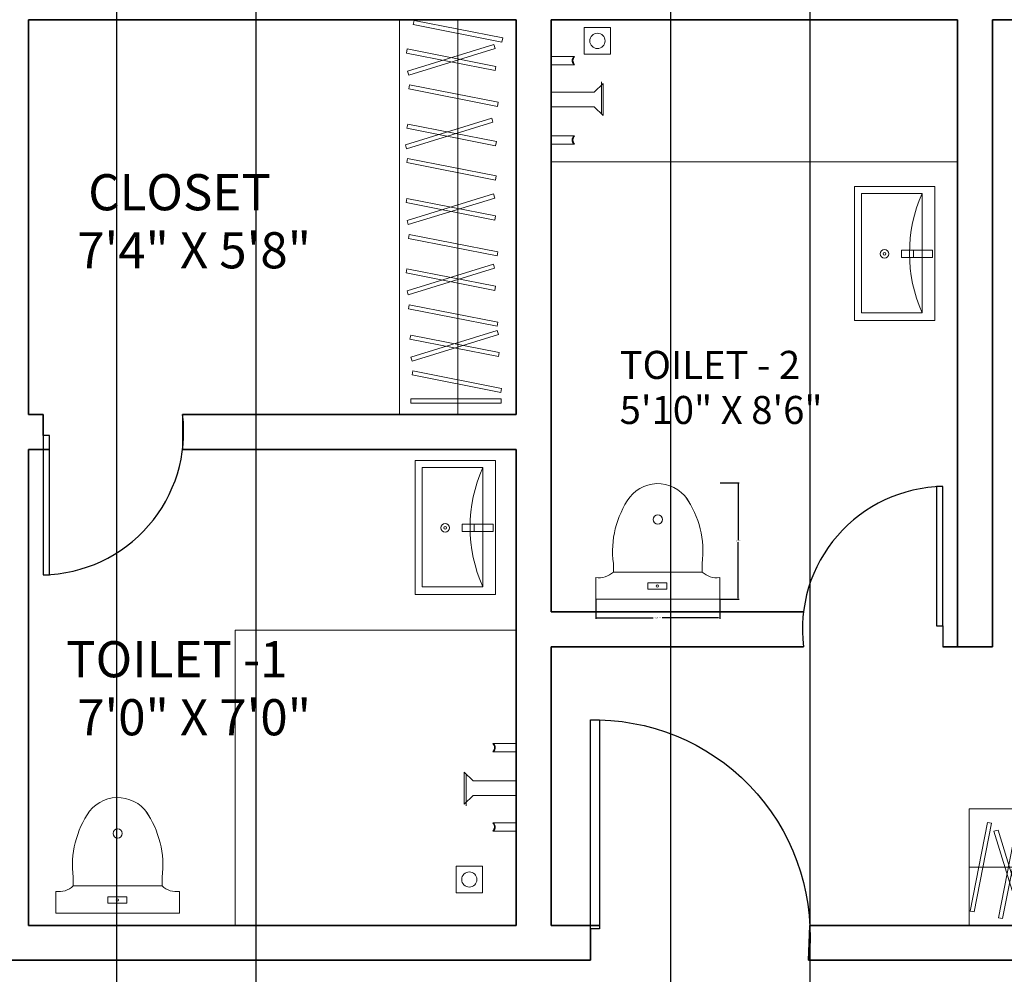
# Model space of a CAD drawing. Units: inches. Extents: x -61 to 1599, y -1316 to 257.
# Tile 141 of 204: x 236 to 406, y -16 to 149. Entities that reach past the tile are written whole.
import ezdxf

# ---------------------------------------------------------------- set-up
doc = ezdxf.new("R2010")
doc.units = ezdxf.units.IN
doc.header["$MEASUREMENT"] = 0
doc.linetypes.add('ACAD_ISO02W100', pattern=[15, 12, -3])
for name, color, linetype, lineweight in [('A-ANNO-DIMS', 2, 'Continuous', 18), ('A-AREA-IDEN', 1, 'Continuous', 18), ('A-FLOR-CASE', 8, 'Continuous', 18), ('A-FLOR-FIXT', 8, 'Continuous', 18), ('A-WALL-JAMB', 4, 'ACAD_ISO02W100', 25), ('DOORS', 2, 'Continuous', 25), ('WALLS', 4, 'Continuous', 35)]:
    doc.layers.add(name, color=color, linetype=linetype, lineweight=lineweight)
doc.styles.get("Standard").update_dxf_attribs({"font": 'arial.ttf'})
doc.dimstyles.get("Standard").update_dxf_attribs({"dimtxt": 0.18, "dimasz": 0.18, "dimexe": 0.18, "dimexo": 0.0625, "dimgap": 0.09, "dimtad": 0, "dimtih": 1, "dimtoh": 1, "dimdec": 0, "dimzin": 0, "dimdsep": 46, "dimlunit": 3, "dimtxsty": 'Standard', "dimcen": 0.09, "dimadec": 0, "dimazin": 0, "dimtfac": 1, "dimtdec": 0, "dimtofl": 0, "dimtmove": 0, "dimatfit": 3, "dimfxl": 1, "dimtolj": 1, "dimtzin": 0, "dimarcsym": 0})

# ---------------------------------------------------------------- blocks, each defined once
blk = doc.blocks.new('DOOR-SWING-24')
blk.add_line((0, 0), (0, 3.6))
blk.add_lwpolyline([(0, 0), (0, -24), (1.05, -24), (1.05, 0)], close=True)
blk.add_arc((-0.44, 0.62), 24.62, 271.0259, 6.9559)
blk = doc.blocks.new('DOOR-SWING-36')
blk.add_line((0, 0), (0, -5.4))
blk.add_lwpolyline([(0, 0), (0, 36), (-1.57, 36), (-1.57, 0)], close=True)
blk.add_arc((-0.74, -1.08), 37.09, 91.2913, 186.6905)
blk = doc.blocks.new('WC-FLOOR-MOUNT')
for p, q in [((3.02, 4.69), (3.02, 6.17)), ((18.31, 4.69), (18.31, 6.17)), ((0, 0), (0, 3.75)), ((3.02, 4.69), (18.31, 4.69)), ((21.33, 0), (21.33, 3.75)), ((0, 0), (21.33, 0))]:
    blk.add_line(p, q)
blk.add_lwpolyline([(12.24, 1.73), (8.96, 1.73), (8.96, 2.81), (12.24, 2.81)], close=True)
for centre, radius in [((10.67, 13.73), 0.792), ((10.6, 2.27), 0.208)]:
    blk.add_circle(centre, radius)
for centre, radius, start, end in [((10.67, 13.73), 6.18, 27.6844, 141.4697), ((19.05, 8.26), 16.17, 144.824, 187.4232), ((2.28, 8.26), 16.17, 352.5768, 35.176), ((0.56, 7.25), 3.55, 260.8586, 313.6993), ((20.77, 7.25), 3.55, 226.3007, 279.1414)]:
    blk.add_arc(centre, radius, start, end)
blk = doc.blocks.new('LAVATORY-WALL')
blk.add_line((10.19, 12.11), (10.19, 10.88))
for points in [[(13.87, 0), (0, 0), (0, 23.07), (13.87, 23.07)], [(13.87, 0), (0, 0), (0, 23.07), (13.87, 23.07)], [(1.2, 1.34), (1.2, 21.88), (11.67, 21.88), (11.67, 1.34)], [(8.09, 10.88), (8.09, 12.11), (13.47, 12.11), (13.47, 10.88)]]:
    blk.add_lwpolyline(points, close=True)
for radius in [0.74, 0.233]:
    blk.add_circle((5.16, 11.5), radius)
blk.add_arc((34.73, 11.61), 25.25, 155.9939, 204.0061)
blk = doc.blocks.new('SHOWER-FITTINGS')
for p, q in [((10.35, 25.72), (6.31, 25.72)), ((10.35, 24.3), (6.31, 24.3)), ((10.35, 23), (10.35, 23)), ((2.92, 19.29), (1.4, 20.76)), ((1.4, 15.27), (1.4, 20.76)), ((1.69, 14.98), (1.69, 20.48)), ((10.35, 19.29), (2.92, 19.29)), ((2.92, 16.74), (1.4, 15.27)), ((10.35, 16.74), (2.92, 16.74)), ((10.35, 12.03), (6.31, 12.03)), ((10.35, 10.61), (6.31, 10.61))]:
    blk.add_line(p, q)
blk.add_lwpolyline([(4.52, 0), (0, 0), (0, 4.57), (4.52, 4.57)], close=True)
blk.add_circle((2.26, 2.29), 1.31)
for points in [[(6.31, 24.3), (6.45, 24.53), (6.75, 25), (6.46, 25.48), (6.31, 25.72)], [(6.45, 24.3), (6.59, 24.53), (6.88, 25), (6.59, 25.48), (6.45, 25.72)], [(6.31, 10.61), (6.45, 10.84), (6.75, 11.31), (6.46, 11.78), (6.31, 12.03)], [(6.45, 10.61), (6.59, 10.84), (6.88, 11.31), (6.59, 11.78), (6.45, 12.03)]]:
    blk.add_open_spline(points, degree=3, knots=[0, 0, 0, 0, 0.7501, 1.532449, 1.532449, 1.532449, 1.532449])
blk = doc.blocks.new('SHOWER-FITTINGS-2')
for p, q in [((0, 15.11), (4.04, 15.11)), ((0, 13.69), (4.04, 13.69)), ((7.43, 8.98), (8.95, 10.45)), ((8.66, 10.73), (8.66, 5.24)), ((8.95, 10.45), (8.95, 4.96)), ((0, 8.98), (7.43, 8.98)), ((0, 6.43), (7.43, 6.43)), ((7.43, 6.43), (8.95, 4.96)), ((0, 1.42), (4.04, 1.42)), ((0, 0), (4.04, 0))]:
    blk.add_line(p, q)
blk.add_lwpolyline([(10.23, 15.5), (5.71, 15.5), (5.71, 20.08), (10.23, 20.08)], close=True)
blk.add_circle((7.97, 17.79), 1.31)
for points in [[(3.91, 15.11), (3.76, 14.88), (3.47, 14.41), (3.76, 13.94), (3.91, 13.69)], [(4.04, 15.11), (3.9, 14.88), (3.6, 14.41), (3.89, 13.94), (4.04, 13.69)], [(3.91, 1.42), (3.76, 1.19), (3.47, 0.72), (3.76, 0.24), (3.91, 0)], [(4.04, 1.42), (3.9, 1.19), (3.6, 0.72), (3.89, 0.24), (4.04, 0)]]:
    blk.add_open_spline(points, degree=3, knots=[0, 0, 0, 0, 0.7501, 1.532449, 1.532449, 1.532449, 1.532449])
blk = doc.blocks.new('WARDROBE-HANGING')
blk.add_line((10.05, 0), (10.05, 68))
for points in [[(20.09, 0), (0, 0), (0, 68), (20.09, 68)], [(2.48, 67.85), (17.75, 64.85), (17.61, 64.14), (2.34, 67.15)], [(1.32, 62.96), (16.59, 59.95), (16.45, 59.25), (1.19, 62.25)], [(1.35, 59.16), (16.22, 63.73), (16.43, 63.04), (1.56, 58.47)], [(1.71, 56.78), (16.98, 53.78), (16.84, 53.07), (1.57, 56.08)], [(1, 46.47), (15.87, 51.04), (16.08, 50.35), (1.21, 45.78)], [(1.39, 50.01), (16.66, 47.01), (16.52, 46.3), (1.26, 49.31)], [(1.36, 44.09), (16.63, 41.09), (16.49, 40.38), (1.23, 43.38)], [(1.28, 33.41), (16.16, 37.98), (16.37, 37.29), (1.49, 32.72)], [(1.26, 37.2), (16.53, 34.2), (16.39, 33.49), (1.12, 36.5)], [(1.65, 31.03), (16.92, 28.03), (16.78, 27.32), (1.51, 30.32)], [(1.28, 21.3), (16.15, 25.87), (16.36, 25.18), (1.49, 20.61)], [(1.26, 25.09), (16.53, 22.09), (16.39, 21.38), (1.12, 24.39)], [(1.65, 18.92), (16.91, 15.92), (16.78, 15.21), (1.51, 18.21)], [(1.91, 13.69), (17.17, 10.68), (17.04, 9.98), (1.77, 12.98)], [(1.93, 9.89), (16.8, 14.46), (17.01, 13.77), (2.14, 9.2)], [(2.29, 7.51), (17.56, 4.51), (17.42, 3.8), (2.16, 6.81)], [(17.49, 1.96), (1.93, 1.96), (1.93, 2.68), (17.49, 2.68)]]:
    blk.add_lwpolyline(points, close=True)
blk = doc.blocks.new('*D616')
at = {"layer": 'A-ANNO-DIMS', "color": 0, "lineweight": -2, "transparency": 16777216}
for p, q in [((335.4, 48.8), (335.4, 45.48)), ((356.73, 48.8), (356.73, 45.48)), ((335.58, 45.66), (345.29, 45.66)), ((356.55, 45.66), (346.84, 45.66))]:
    blk.add_line(p, q, dxfattribs=at)
at = {"layer": 'A-ANNO-DIMS', "color": 0, "transparency": 16777216}
for points in [[(335.58, 45.69), (335.58, 45.63), (335.4, 45.66)], [(356.55, 45.69), (356.55, 45.63), (356.73, 45.66)]]:
    blk.add_solid(points, dxfattribs=at)
at = {"layer": 'DEFPOINTS', "color": 0, "transparency": 16777216}
for p in [(335.4, 48.86), (356.73, 48.86), (356.73, 45.66)]:
    blk.add_point(p, dxfattribs=at)
at = {"layer": 'A-ANNO-DIMS', "color": 0, "transparency": 16777216, "insert": (346.07, 45.66), "char_height": 0.18, "attachment_point": 5}
blk.add_mtext('\\A1;WC 21 TYP.', dxfattribs=at)
blk = doc.blocks.new('*D617')
at = {"layer": 'A-ANNO-DIMS', "color": 0, "lineweight": -2, "transparency": 16777216}
for p, q in [((356.8, 68.94), (360.11, 68.94)), ((359.93, 68.76), (359.93, 59.08)), ((359.93, 49.04), (359.93, 58.72)), ((356.8, 48.86), (360.11, 48.86))]:
    blk.add_line(p, q, dxfattribs=at)
at = {"layer": 'A-ANNO-DIMS', "color": 0, "transparency": 16777216}
for points in [[(359.9, 68.76), (359.96, 68.76), (359.93, 68.94)], [(359.9, 49.04), (359.96, 49.04), (359.93, 48.86)]]:
    blk.add_solid(points, dxfattribs=at)
at = {"layer": 'DEFPOINTS', "color": 0, "transparency": 16777216}
for p in [(356.73, 68.94), (359.93, 68.94), (356.73, 48.86)]:
    blk.add_point(p, dxfattribs=at)
at = {"layer": 'A-ANNO-DIMS', "color": 0, "transparency": 16777216, "insert": (359.93, 58.9), "char_height": 0.18, "attachment_point": 5}
blk.add_mtext('\\A1;20 TYP.', dxfattribs=at)
blk = doc.blocks.new('*D687')
at = {"layer": 'A-ANNO-DIMS', "color": 0, "lineweight": -2, "transparency": 16777216}
for p, q in [((289.42, 181.68), (-61.08, 181.68)), ((-60.9, 181.5), (-60.9, -528.95)), ((-60.9, -1239.76), (-60.9, -529.32)), ((319.64, -1239.94), (-61.08, -1239.94))]:
    blk.add_line(p, q, dxfattribs=at)
at = {"layer": 'A-ANNO-DIMS', "color": 0, "transparency": 16777216}
for points in [[(-60.93, 181.5), (-60.87, 181.5), (-60.9, 181.68)], [(-60.93, -1239.76), (-60.87, -1239.76), (-60.9, -1239.94)]]:
    blk.add_solid(points, dxfattribs=at)
at = {"layer": 'DEFPOINTS', "color": 0, "transparency": 16777216}
for p in [(289.48, 181.68), (-60.9, -1239.94), (319.7, -1239.94)]:
    blk.add_point(p, dxfattribs=at)
at = {"layer": 'A-ANNO-DIMS', "color": 0, "transparency": 16777216, "insert": (-60.9, -529.13), "char_height": 0.18, "attachment_point": 5}
blk.add_mtext('\\A1;1421.6', dxfattribs=at)
blk = doc.blocks.new('*D701')
at = {"layer": 'A-ANNO-DIMS', "color": 0, "lineweight": -2, "transparency": 16777216}
for p, q in [((215.75, -616.88), (215.75, 257.46)), ((215.93, 257.28), (233.92, 257.28)), ((252.7, 257.28), (234.71, 257.28)), ((252.88, -616.88), (252.88, 257.46))]:
    blk.add_line(p, q, dxfattribs=at)
at = {"layer": 'A-ANNO-DIMS', "color": 0, "transparency": 16777216}
for points in [[(215.93, 257.31), (215.93, 257.25), (215.75, 257.28)], [(252.7, 257.31), (252.7, 257.25), (252.88, 257.28)]]:
    blk.add_solid(points, dxfattribs=at)
at = {"layer": 'DEFPOINTS', "color": 0, "transparency": 16777216}
for p in [(252.88, 257.28), (215.75, -616.94), (252.88, -616.94)]:
    blk.add_point(p, dxfattribs=at)
at = {"layer": 'A-ANNO-DIMS', "color": 0, "transparency": 16777216, "insert": (234.32, 257.28), "char_height": 0.18, "attachment_point": 5}
blk.add_mtext('\\A1;37.13', dxfattribs=at)
blk = doc.blocks.new('*D702')
at = {"layer": 'A-ANNO-DIMS', "color": 0, "lineweight": -2, "transparency": 16777216}
for p, q in [((276.88, -616.88), (276.88, 257.46)), ((277.06, 257.28), (312.21, 257.28)), ((348.14, 257.28), (312.99, 257.28)), ((348.32, -616.88), (348.32, 257.46))]:
    blk.add_line(p, q, dxfattribs=at)
at = {"layer": 'A-ANNO-DIMS', "color": 0, "transparency": 16777216}
for points in [[(277.06, 257.31), (277.06, 257.25), (276.88, 257.28)], [(348.14, 257.31), (348.14, 257.25), (348.32, 257.28)]]:
    blk.add_solid(points, dxfattribs=at)
at = {"layer": 'DEFPOINTS', "color": 0, "transparency": 16777216}
for p in [(348.32, 257.28), (276.88, -616.94), (348.32, -616.94)]:
    blk.add_point(p, dxfattribs=at)
at = {"layer": 'A-ANNO-DIMS', "color": 0, "transparency": 16777216, "insert": (312.6, 257.28), "char_height": 0.18, "attachment_point": 5}
blk.add_mtext('\\A1;71.44', dxfattribs=at)
blk = doc.blocks.new('*D703')
at = {"layer": 'A-ANNO-DIMS', "color": 0, "lineweight": -2, "transparency": 16777216}
for p, q in [((372.32, -616.88), (372.32, 257.46)), ((372.5, 257.28), (413.7, 257.28)), ((455.65, 257.28), (414.45, 257.28)), ((455.83, -616.88), (455.83, 257.46))]:
    blk.add_line(p, q, dxfattribs=at)
at = {"layer": 'A-ANNO-DIMS', "color": 0, "transparency": 16777216}
for points in [[(372.5, 257.31), (372.5, 257.25), (372.32, 257.28)], [(455.65, 257.31), (455.65, 257.25), (455.83, 257.28)]]:
    blk.add_solid(points, dxfattribs=at)
at = {"layer": 'DEFPOINTS', "color": 0, "transparency": 16777216}
for p in [(455.83, 257.28), (372.32, -616.94), (455.83, -616.94)]:
    blk.add_point(p, dxfattribs=at)
at = {"layer": 'A-ANNO-DIMS', "color": 0, "transparency": 16777216, "insert": (414.08, 257.28), "char_height": 0.18, "attachment_point": 5}
blk.add_mtext('\\A1;83.51', dxfattribs=at)

msp = doc.modelspace()

# ---------------------------------------------------------------- linework, layer by layer
at = {"layer": 'A-FLOR-FIXT'}
for p, q in [((327.7028, 124.2077), (397.7028, 124.2077)), ((321.7028, 43.5315), (273.2827, 43.5315)), ((273.2827, 43.5315), (273.2827, -7.3229))]:
    msp.add_line(p, q, dxfattribs=at)
at = {"layer": 'A-WALL-JAMB'}
for p, q in [((240.2351, 80.6771), (240.2351, 74.6771)), ((264.2351, 80.6771), (264.2306, 74.6771)), ((334.4752, -13.3229), (334.4752, -7.3229)), ((372.0502, -13.3229), (372.2648, -7.3229))]:
    msp.add_line(p, q, dxfattribs=at)
at = {"layer": 'WALLS'}
for p, q in [((237.7028, 148.6771), (237.7028, 80.6771)), ((237.7028, 148.6771), (321.7028, 148.6771)), ((321.7028, 148.6771), (321.7028, 80.6771)), ((327.7028, 148.6771), (327.7028, 46.6771)), ((327.7028, 148.6771), (397.7028, 148.6771)), ((397.7028, 148.6771), (397.7028, 40.6771)), ((403.7028, 148.6771), (403.7028, 40.6771)), ((403.7028, 148.6771), (535.7028, 148.6771)), ((237.7028, 80.6771), (240.2351, 80.6771)), ((264.2351, 80.6771), (321.7028, 80.6771)), ((237.7028, 74.6771), (241.2851, 74.6771)), ((237.7028, 74.6771), (237.7028, -7.3229)), ((264.2306, 74.6771), (321.7028, 74.6771)), ((321.7028, 74.6771), (321.7028, -7.3229)), ((327.7028, 46.6771), (371.1506, 46.6771)), ((327.7028, 40.6771), (371.1461, 40.6771)), ((327.7028, 40.6771), (327.7028, -7.3229)), ((395.1461, 40.6771), (403.7028, 40.6771)), ((237.7028, -7.3229), (321.7028, -7.3229)), ((327.7028, -7.3229), (336.0502, -7.3229)), ((372.2648, -7.3229), (403.7028, -7.3229)), ((397.7028, -7.3229), (535.7028, -7.3229)), ((223.0506, -13.3229), (237.7028, -13.3229)), ((237.7028, -13.3229), (327.7028, -13.3229)), ((321.7028, -13.3229), (334.4752, -13.3229)), ((372.0502, -13.3229), (403.7028, -13.3229)), ((397.7028, -13.3229), (535.7028, -13.3229))]:
    msp.add_line(p, q, dxfattribs=at)

# ---------------------------------------------------------------- block references
at = {"layer": 'A-FLOR-CASE'}
msp.add_blockref('WARDROBE-HANGING', (301.609, 80.677), dxfattribs=at)
at = {"layer": 'A-FLOR-CASE', "rotation": 90.00000000000017}
msp.add_blockref('WARDROBE-HANGING', (467.7029, -7.3231), dxfattribs=at)
at = {"layer": 'A-FLOR-FIXT'}
for name, p in [('SHOWER-FITTINGS-2', (327.703, 127.237)), ('LAVATORY-WALL', (379.936, 96.864)), ('LAVATORY-WALL', (304.2705, 49.6634)), ('WC-FLOOR-MOUNT', (335.402, 48.864)), ('SHOWER-FITTINGS', (311.351, -1.689)), ('WC-FLOOR-MOUNT', (242.3826, -5.2012))]:
    msp.add_blockref(name, p, dxfattribs=at)
at = {"layer": 'DOORS'}
msp.add_blockref('DOOR-SWING-24', (240.2351, 77.0771), dxfattribs=at)
at = {"layer": 'DOORS', "rotation": 180}
msp.add_blockref('DOOR-SWING-24', (395.1461, 44.2771), dxfattribs=at)
at = {"layer": 'DOORS', "extrusion": (0, 0, -1), "zscale": -1}
msp.add_blockref('DOOR-SWING-36', (-334.4752, -7.9229), dxfattribs=at)

# ---------------------------------------------------------------- texts
at = {"layer": 'A-AREA-IDEN'}
for s, height, p in [('   CLOSET', 6.22364, (242.2634, 115.8502)), ('  7\'4" X 5\'8"', 6.223643, (242.2634, 105.8525)), ('TOILET - 2', 4.8321, (339.5043, 86.8095)), ('5\'10" X 8\'6"', 4.832098, (339.5043, 79.0472)), (' TOILET -1', 6.22364, (242.2634, 35.4228)), ('  7\'0" X 7\'0"', 6.223643, (242.2634, 25.425))]:
    msp.add_text(s, height=height, dxfattribs=at).set_placement(p)

# ---------------------------------------------------------------- dimensions: what is measured, and where the dimension line sits
at = {"layer": 'A-ANNO-DIMS'}
for base, p1, p2, picture, middle in [((252.8825, 257.2771), (215.7521, -616.9446), (252.8825, -616.9446), '*D701', (234.3173, 257.2771)), ((348.3201, 257.2771), (276.8825, -616.9446), (348.3201, -616.9446), '*D702', (312.6013, 257.2771)), ((455.8327, 257.2771), (372.3201, -616.9446), (455.8327, -616.9446), '*D703', (414.0764, 257.2771))]:
    dim = msp.add_linear_dim(base=base, p1=p1, p2=p2, dimstyle='Standard', override={"dimdec": 2, "dimlfac": 1, "dimrnd": 0, "dimzin": 0, "dimdsep": 46, "dimlunit": 2}, dxfattribs=at)
    dim.commit()
    dim.dimension.update_dxf_attribs({"geometry": picture, "text_midpoint": middle})
dim = msp.add_linear_dim(base=(-60.8972, -1239.9446), p1=(289.4807, 181.6771), p2=(319.7028, -1239.9446), angle=90, dimstyle='Standard', override={"dimdec": 1, "dimlfac": 1, "dimrnd": 0, "dimzin": 0, "dimdsep": 46, "dimlunit": 2}, dxfattribs=at)
dim.commit()
dim.dimension.update_dxf_attribs({"geometry": '*D687', "text_midpoint": (-60.8972, -529.1337)})
dim = msp.add_linear_dim(base=(359.9329, 68.9385), p1=(356.7333, 48.8644), p2=(356.7333, 68.9385), angle=90, text='<> TYP.', dimstyle='Standard', override={"dimdec": 0, "dimlfac": 1, "dimrnd": 0, "dimzin": 0, "dimdsep": 46, "dimlunit": 2}, dxfattribs=at)
dim.commit()
dim.dimension.update_dxf_attribs({"geometry": '*D617', "text_midpoint": (359.9329, 58.9015)})
dim = msp.add_linear_dim(base=(356.7333, 45.6648), p1=(335.4025, 48.8644), p2=(356.7333, 48.8644), text='WC <> TYP.', dimstyle='Standard', override={"dimdec": 0, "dimlfac": 1, "dimrnd": 0, "dimzin": 0, "dimdsep": 46, "dimlunit": 2}, dxfattribs=at)
dim.commit()
dim.dimension.update_dxf_attribs({"geometry": '*D616', "text_midpoint": (346.0679, 45.6648)})

doc.saveas('drawing.dxf')
